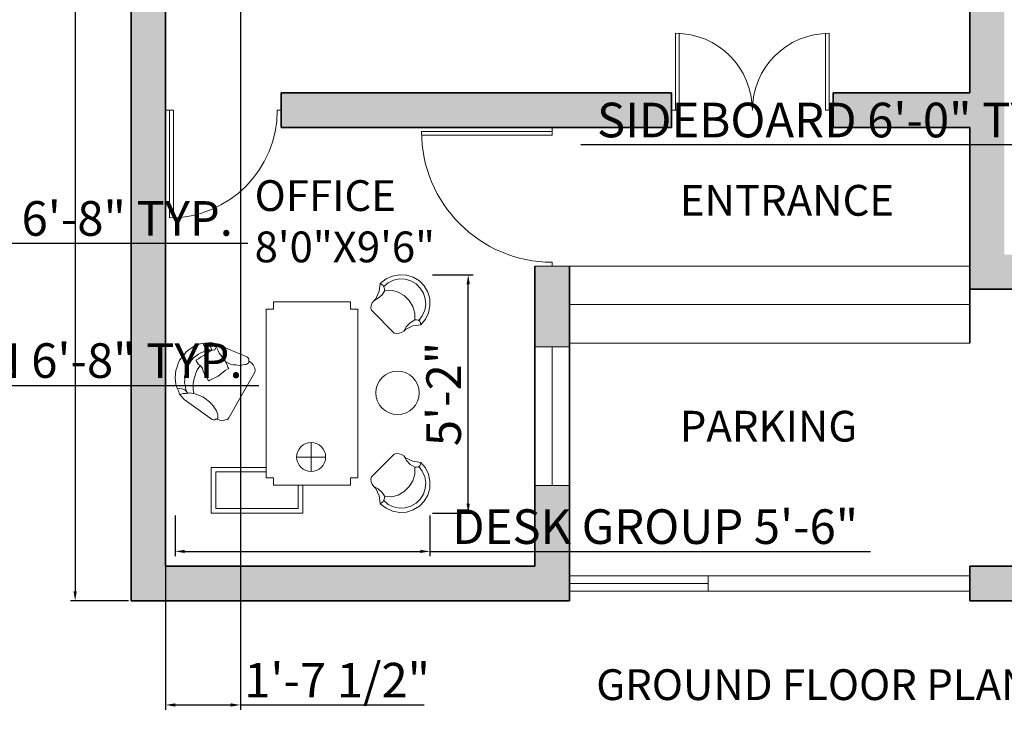
# Model space of a CAD drawing. Units: inches. Extents: x 3592 to 4861, y 1650 to 2243.
# Tile 2 of 30: x 4009 to 4265, y 1650 to 1836. Entities that reach past the tile are written whole.
import ezdxf

# ---------------------------------------------------------------- set-up
doc = ezdxf.new("R2010")
doc.units = ezdxf.units.IN
for name, color, linetype, lineweight in [('A-ANNO-DIMS', 2, 'Continuous', 13), ('A-ANNO-TEXT', 7, 'Continuous', 25), ('A-AREA-IDEN', 7, 'Continuous', 18), ('A-DOOR', 3, 'Continuous', 20), ('A-FLOR-STRS', 7, 'Continuous', 18), ('A-FURN', 9, 'Continuous', 13), ('A-GLAZ', 4, 'Continuous', 18), ('A-WALL', 7, 'Continuous', 35)]:
    doc.layers.add(name, color=color, linetype=linetype, lineweight=lineweight)
doc.layers.add('A-WALL-PATT', color=252, linetype='Continuous', lineweight=13, true_color=0x939598)
doc.styles.get("Standard").update_dxf_attribs({"font": 'arial.ttf'})
doc.dimstyles.new('ISO-25', dxfattribs={"dimtxt": 9, "dimasz": 2.5, "dimexe": 1.25, "dimexo": 0.625, "dimtad": 1, "dimlunit": 3, "dimtxsty": 'Standard', "dimcen": 2.5, "dimadec": 0, "dimazin": 0, "dimtfac": 1, "dimtmove": 0, "dimatfit": 3, "dimfxl": 1, "dimarcsym": 0})

# ---------------------------------------------------------------- blocks, each defined once
blk = doc.blocks.new('2')
for p, q in [((3637.19, 1914.49), (3637.19, 1942.49)), ((3638.19, 1914.49), (3638.19, 1942.49)), ((3636.19, 1914.49), (3638.19, 1914.49)), ((3665.19, 1914.49), (3666.19, 1914.49))]:
    blk.add_line(p, q)
blk.add_arc((3637.19, 1914.49), 28, 0, 90)
blk = doc.blocks.new('1')
for p, q in [((3628.27, 1890.86), (3628.27, 1924.86)), ((3629.27, 1890.86), (3629.27, 1924.86)), ((3627.27, 1890.86), (3629.27, 1890.86)), ((3662.27, 1890.86), (3663.27, 1890.86))]:
    blk.add_line(p, q)
blk.add_arc((3628.27, 1890.86), 34, 0, 90)
blk = doc.blocks.new('MD')
for p, q in [((3665.34, 1831.69), (3665.34, 1851.69)), ((3666.34, 1831.69), (3666.34, 1851.69)), ((3704.34, 1831.69), (3704.34, 1851.69)), ((3705.34, 1831.69), (3705.34, 1851.69)), ((3664.34, 1831.69), (3666.34, 1831.69)), ((3706.34, 1831.69), (3704.34, 1831.69))]:
    blk.add_line(p, q)
for centre, start, end in [((3665.34, 1831.69), 0, 90), ((3705.34, 1831.69), 90, 180)]:
    blk.add_arc(centre, 20, start, end)
blk = doc.blocks.new('*D6')
at = {"layer": 'A-ANNO-DIMS', "color": 0, "lineweight": -2, "transparency": 16777216}
for p, q in [((4037.74, 2165.22), (4022.59, 2165.22)), ((4023.84, 2162.72), (4023.84, 1687.72)), ((4037.74, 1685.22), (4022.59, 1685.22))]:
    blk.add_line(p, q, dxfattribs=at)
at = {"layer": 'A-ANNO-DIMS', "color": 0, "transparency": 16777216}
for points in [[(4023.43, 2162.72), (4024.26, 2162.72), (4023.84, 2165.22)], [(4023.43, 1687.72), (4024.26, 1687.72), (4023.84, 1685.22)]]:
    blk.add_solid(points, dxfattribs=at)
at = {"layer": 'Defpoints', "color": 0, "transparency": 16777216}
for p in [(4038.37, 2165.22), (4023.84, 1685.22), (4038.37, 1685.22)]:
    blk.add_point(p, dxfattribs=at)
at = {"layer": 'A-ANNO-DIMS', "color": 0, "transparency": 16777216, "insert": (4018.62, 1925.22), "char_height": 9, "attachment_point": 5, "rotation": 90}
blk.add_mtext("40'", dxfattribs=at)
blk = doc.blocks.new('desk-20')
at = {"color": 0, "linetype": 'ByBlock'}
for p, q in [((0.2166, 1.9076), (0.1582, 1.8904)), ((0.2792, 1.9099), (0.2166, 1.9076)), ((0.3395, 1.8969), (0.2792, 1.9099)), ((0.3961, 1.8709), (0.3395, 1.8969)), ((1.6928, 1.8709), (1.7493, 1.8969)), ((1.7493, 1.8969), (1.8096, 1.9099)), ((1.8096, 1.9099), (1.8723, 1.9076)), ((1.8723, 1.9076), (1.9307, 1.8904)), ((0.0616, 1.8175), (0.0287, 1.7633)), ((0.1043, 1.8602), (0.0616, 1.8175)), ((0.1238, 1.8255), (0.0875, 1.7892)), ((0.1582, 1.8904), (0.1043, 1.8602)), ((0.167, 1.8534), (0.1238, 1.8255)), ((0.2166, 1.8686), (0.167, 1.8534)), ((0.2662, 1.8732), (0.2166, 1.8686)), ((0.3178, 1.8644), (0.2662, 1.8732)), ((0.3655, 1.8427), (0.3178, 1.8644)), ((0.4064, 1.8125), (0.3655, 1.8427)), ((0.4434, 1.8297), (0.3961, 1.8709)), ((0.4045, 1.8083), (0.4003, 1.7934)), ((0.4129, 1.8213), (0.4045, 1.8083)), ((0.4285, 1.8278), (0.4129, 1.8213)), ((0.4434, 1.8297), (0.4285, 1.8278)), ((0.4434, 1.8297), (0.4537, 1.7591)), ((1.6455, 1.8297), (1.6351, 1.7591)), ((1.6455, 1.8297), (1.6928, 1.8709)), ((1.6455, 1.8297), (1.6604, 1.8278)), ((1.6604, 1.8278), (1.676, 1.8213)), ((1.676, 1.8213), (1.6844, 1.8083)), ((1.6825, 1.8125), (1.7234, 1.8427)), ((1.6844, 1.8083), (1.6886, 1.7934)), ((1.7234, 1.8427), (1.7711, 1.8644)), ((1.7711, 1.8644), (1.8226, 1.8732)), ((1.8226, 1.8732), (1.8723, 1.8686)), ((1.8723, 1.8686), (1.9219, 1.8534)), ((1.9219, 1.8534), (1.9651, 1.8255)), ((1.9307, 1.8904), (1.9845, 1.8602)), ((1.9651, 1.8255), (2.0013, 1.7892)), ((1.9845, 1.8602), (2.0273, 1.8175)), ((2.0273, 1.8175), (2.0601, 1.7633)), ((0.0287, 1.7633), (0.0096, 1.7052)), ((0.0612, 1.7438), (0.0463, 1.6945)), ((0.0875, 1.7892), (0.0612, 1.7438)), ((0.2315, 1.7285), (0.1887, 1.6857)), ((0.2834, 1.7606), (0.2315, 1.7285)), ((0.3418, 1.7762), (0.2834, 1.7606)), ((0.4022, 1.7785), (0.3418, 1.7762)), ((0.4003, 1.7934), (0.4022, 1.7785)), ((0.4022, 1.7785), (0.4258, 1.7373)), ((0.4258, 1.7373), (0.4602, 1.7052)), ((0.4537, 1.7591), (0.4843, 1.6964)), ((1.6351, 1.7591), (1.6046, 1.6964)), ((1.663, 1.7373), (1.6287, 1.7052)), ((1.6867, 1.7785), (1.663, 1.7373)), ((1.6886, 1.7934), (1.6867, 1.7785)), ((1.6867, 1.7785), (1.747, 1.7762)), ((1.747, 1.7762), (1.8054, 1.7606)), ((1.8054, 1.7606), (1.8574, 1.7285)), ((1.8574, 1.7285), (1.9001, 1.6857)), ((2.0013, 1.7892), (2.0277, 1.7438)), ((2.0277, 1.7438), (2.0426, 1.6945)), ((2.0601, 1.7633), (2.0792, 1.7052)), ((0.0096, 1.7052), (0.0073, 1.6426)), ((0.0073, 1.6426), (0.0184, 1.5819)), ((0.0463, 1.6945), (0.0444, 1.6422)), ((0.0444, 1.6422), (0.0551, 1.5926)), ((0.1887, 1.6857), (0.1586, 1.6334)), ((0.4602, 1.7052), (0.5011, 1.6812)), ((0.5011, 1.6812), (0.4843, 1.6964)), ((0.5121, 1.6617), (0.5011, 1.6812)), ((0.5186, 1.6399), (0.5121, 1.6617)), ((0.5209, 1.6185), (0.5186, 1.6399)), ((1.5679, 1.6185), (1.5702, 1.6399)), ((1.5702, 1.6399), (1.5767, 1.6617)), ((1.5767, 1.6617), (1.5878, 1.6812)), ((1.6287, 1.7052), (1.5878, 1.6812)), ((1.5878, 1.6812), (1.6046, 1.6964)), ((1.9001, 1.6857), (1.9303, 1.6334)), ((2.0445, 1.6422), (2.0338, 1.5926)), ((2.0426, 1.6945), (2.0445, 1.6422)), ((2.0815, 1.6426), (2.0704, 1.5819)), ((2.0792, 1.7052), (2.0815, 1.6426)), ((0.0184, 1.5819), (0.044, 1.5258)), ((0.0551, 1.5926), (0.0765, 1.5452)), ((0.1586, 1.6334), (0.1433, 1.5754)), ((0.1433, 1.5754), (0.1452, 1.5154)), ((0.5163, 1.5972), (0.3174, 1.3982)), ((0.5163, 1.5972), (0.5209, 1.6185)), ((1.5725, 1.5972), (1.5679, 1.6185)), ((1.5725, 1.5972), (1.7715, 1.3982)), ((1.9303, 1.6334), (1.9456, 1.5754)), ((1.9456, 1.5754), (1.9437, 1.5154)), ((2.0338, 1.5926), (2.0124, 1.5452)), ((2.0704, 1.5819), (2.0449, 1.5258)), ((0.044, 1.5258), (0.0829, 1.4761)), ((0.0765, 1.5452), (0.1108, 1.5063)), ((0.0982, 1.4975), (0.0829, 1.4761)), ((0.1517, 1.4654), (0.0829, 1.4761)), ((0.1196, 1.5105), (0.0982, 1.4975)), ((0.1452, 1.5154), (0.1196, 1.5105)), ((0.1818, 1.4918), (0.1452, 1.5154)), ((0.2166, 1.4356), (0.1517, 1.4654)), ((0.212, 1.457), (0.1818, 1.4918)), ((1.8723, 1.4356), (1.9372, 1.4654)), ((1.8769, 1.457), (1.907, 1.4918)), ((1.907, 1.4918), (1.9437, 1.5154)), ((1.9372, 1.4654), (2.0059, 1.4761)), ((1.9437, 1.5154), (1.9693, 1.5105)), ((1.9693, 1.5105), (1.9906, 1.4975)), ((2.0124, 1.5452), (1.978, 1.5063)), ((1.9906, 1.4975), (2.0059, 1.4761)), ((2.0449, 1.5258), (2.0059, 1.4761)), ((0.2342, 1.4181), (0.212, 1.457)), ((0.2166, 1.4356), (0.2342, 1.4181)), ((0.2342, 1.4181), (0.2532, 1.4051)), ((0.2532, 1.4051), (0.275, 1.3963)), ((0.275, 1.3963), (0.2983, 1.3944)), ((0.2983, 1.3944), (0.3174, 1.3982)), ((1.7906, 1.3944), (1.7715, 1.3982)), ((1.8138, 1.3963), (1.7906, 1.3944)), ((1.8356, 1.4051), (1.8138, 1.3963)), ((1.8547, 1.4181), (1.8356, 1.4051)), ((1.8547, 1.4181), (1.8769, 1.457)), ((1.8723, 1.4356), (1.8547, 1.4181)), ((0.3084, 1.2145), (0.2444, 1.2145)), ((0.2444, 1.2145), (0.2444, 0.5425)), ((0.3084, 1.2785), (0.3084, 1.2145)), ((1.7804, 1.2785), (0.3084, 1.2785)), ((1.7804, 1.2145), (1.7804, 1.2785)), ((1.8444, 1.2145), (1.7804, 1.2145)), ((1.8444, 0.5425), (1.8444, 1.2145)), ((0.4901, 0.7453), (0.4901, 0.9986)), ((0.6167, 0.8719), (0.3635, 0.8719)), ((0.2444, 0.8), (0, 0.8)), ((0, 0.8), (0, 0)), ((0.2444, 0.76), (0.04, 0.76)), ((0.04, 0.76), (0.04, 0.04)), ((0.2444, 0.5425), (0.3084, 0.5425)), ((0.3084, 0.5425), (0.3084, 0.4785)), ((1.7804, 0.4785), (1.7804, 0.5425)), ((1.7804, 0.5425), (1.8444, 0.5425)), ((0.3084, 0.4785), (1.7804, 0.4785)), ((0.36, 0.04), (0.36, 0.4785)), ((0.4, 0), (0.4, 0.4785)), ((1.2309, 0.3814), (0.831, 0.1524)), ((0.831, 0.1524), (1.2309, 0.3814)), ((1.2309, 0.3814), (1.2494, 0.3818)), ((1.2309, 0.3814), (1.2494, 0.3818)), ((1.2494, 0.3818), (1.2673, 0.3798)), ((1.2494, 0.3818), (1.2673, 0.3798)), ((1.2673, 0.3798), (1.2823, 0.3718)), ((1.2673, 0.3798), (1.2823, 0.3718)), ((1.2823, 0.3718), (1.2955, 0.3671)), ((1.2823, 0.3718), (1.2955, 0.3671)), ((1.2955, 0.3671), (1.3075, 0.3573)), ((1.2955, 0.3671), (1.3075, 0.3573)), ((1.3075, 0.3573), (1.3196, 0.3436)), ((1.3075, 0.3573), (1.3196, 0.3436)), ((1.2931, 0.2677), (1.2906, 0.2433)), ((1.2971, 0.2929), (1.2931, 0.2677)), ((1.2988, 0.3043), (1.2971, 0.2929)), ((1.3007, 0.3117), (1.2988, 0.3043)), ((1.3076, 0.3178), (1.3007, 0.3117)), ((1.3104, 0.3236), (1.3076, 0.3178)), ((1.3191, 0.3266), (1.3104, 0.3236)), ((1.3262, 0.3287), (1.3191, 0.3266)), ((1.3196, 0.3436), (1.3262, 0.3287)), ((1.3196, 0.3436), (1.3262, 0.3287)), ((1.3392, 0.3279), (1.3262, 0.3287)), ((1.3262, 0.3287), (1.3392, 0.3279)), ((1.3441, 0.3266), (1.3392, 0.3279)), ((1.3392, 0.3279), (1.3441, 0.3266)), ((1.3515, 0.3247), (1.3441, 0.3266)), ((1.3441, 0.3266), (1.3515, 0.3247)), ((1.3582, 0.3203), (1.3515, 0.3247)), ((1.3515, 0.3247), (1.3582, 0.3203)), ((1.3637, 0.3109), (1.3582, 0.3203)), ((1.3582, 0.3203), (1.3637, 0.3109)), ((1.4807, 0.0353), (1.3637, 0.3109)), ((1.3637, 0.3109), (1.4807, 0.0353)), ((1.2906, 0.2433), (1.294, 0.2161)), ((1.294, 0.2161), (1.2946, 0.1936)), ((1.2946, 0.1936), (1.302, 0.1666)), ((0.8074, 0.0928), (0.8104, 0.1091)), ((0.8074, 0.0928), (0.8104, 0.1091)), ((0.8091, 0.0792), (0.8074, 0.0928)), ((0.8091, 0.0792), (0.8074, 0.0928)), ((0.8104, 0.1091), (0.8137, 0.1214)), ((0.8104, 0.1091), (0.8137, 0.1214)), ((0.8137, 0.1214), (0.8173, 0.1402)), ((0.8137, 0.1214), (0.8173, 0.1402)), ((0.8173, 0.1402), (0.831, 0.1524)), ((0.8173, 0.1402), (0.831, 0.1524)), ((1.2452, 0.121), (1.196, 0.059)), ((1.2452, 0.121), (1.2633, 0.1544)), ((1.2633, 0.1544), (1.2752, 0.1447)), ((1.2752, 0.1447), (1.2859, 0.1406)), ((1.3249, 0.1237), (1.2859, 0.1406)), ((1.302, 0.1666), (1.3216, 0.1259)), ((1.3638, 0.0964), (1.3249, 0.1237)), ((1.3971, 0.0679), (1.3638, 0.0964)), ((0, 0), (0.4, 0)), ((0.04, 0.04), (0.36, 0.04)), ((0.8169, 0.0587), (0.8091, 0.0792)), ((0.8169, 0.0587), (0.8091, 0.0792)), ((0.8138, 0.0319), (0.8118, 0.0245)), ((0.8118, 0.0245), (0.8138, 0.0319)), ((0.8118, 0.0245), (0.8155, 0.0183)), ((0.8155, 0.0183), (0.8118, 0.0245)), ((0.8206, 0.038), (0.8138, 0.0319)), ((0.8138, 0.0319), (0.8206, 0.038)), ((0.8155, 0.0183), (0.8178, 0.0072)), ((0.8178, 0.0072), (0.8155, 0.0183)), ((0.8208, 0.0485), (0.8169, 0.0587)), ((0.8208, 0.0485), (0.8169, 0.0587)), ((0.8178, 0.0072), (0.9916, -0.2373)), ((0.9916, -0.2373), (0.8178, 0.0072)), ((0.8208, 0.0485), (0.8206, 0.038)), ((0.8206, 0.038), (0.8208, 0.0485)), ((0.8261, 0.0537), (0.8208, 0.0485)), ((0.8348, 0.0567), (0.8261, 0.0537)), ((0.8444, 0.0581), (0.8348, 0.0567)), ((0.8549, 0.058), (0.8444, 0.0581)), ((0.8613, 0.0576), (0.8549, 0.058)), ((0.8681, 0.0532), (0.8613, 0.0576)), ((0.8936, 0.0451), (0.8681, 0.0532)), ((0.9113, 0.0326), (0.8936, 0.0451)), ((0.9358, 0.0156), (0.9113, 0.0326)), ((0.956, 0.0024), (0.9358, 0.0156)), ((0.9734, -0.0167), (0.956, 0.0024)), ((1.196, 0.059), (1.1611, -0.0135)), ((1.3971, 0.0679), (1.4186, 0.0596)), ((1.4217, 0.0114), (1.4121, -0.0151)), ((1.4186, 0.0596), (1.4462, 0.0444)), ((1.4211, 0.0089), (1.4385, 0.0004)), ((1.4238, 0.0043), (1.4213, -0.0201)), ((1.4217, 0.0114), (1.4262, 0.0286)), ((1.4433, 0.0386), (1.4231, 0.0268)), ((1.4273, -0.0125), (1.4238, 0.0043)), ((1.4385, 0.0004), (1.465, -0.0092)), ((1.4462, 0.0444), (1.4433, 0.0386)), ((1.4865, 0.0075), (1.4807, 0.0353)), ((1.4807, 0.0353), (1.4865, 0.0075)), ((1.4876, -0.0231), (1.4865, 0.0075)), ((1.4865, 0.0075), (1.4876, -0.0231)), ((1.0007, -0.0528), (0.9734, -0.0167)), ((1.015, -0.0737), (1.0007, -0.0528)), ((1.0237, -0.0957), (1.015, -0.0737)), ((1.1552, -0.0211), (1.1611, -0.0135)), ((1.1554, -0.0251), (1.1552, -0.0211)), ((1.1763, -0.0359), (1.1554, -0.0251)), ((1.1911, -0.0398), (1.1763, -0.0359)), ((1.1911, -0.0398), (1.2124, -0.0586)), ((1.2124, -0.0586), (1.2367, -0.0715)), ((1.2367, -0.0715), (1.2653, -0.0777)), ((1.2934, -0.1009), (1.2653, -0.0777)), ((1.3766, -0.0649), (1.3636, -0.0892)), ((1.392, -0.0414), (1.3766, -0.0649)), ((1.4121, -0.0151), (1.392, -0.0414)), ((1.409, -0.0669), (1.4001, -0.0908)), ((1.417, -0.0414), (1.409, -0.0669)), ((1.4213, -0.0201), (1.417, -0.0414)), ((1.4332, -0.0298), (1.4273, -0.0125)), ((1.4441, -0.0485), (1.4332, -0.0298)), ((1.4646, -0.0657), (1.4441, -0.0485)), ((1.4803, -0.0712), (1.4646, -0.0657)), ((1.465, -0.0092), (1.4889, -0.0182)), ((1.4717, -0.1137), (1.4804, -0.0857)), ((1.4804, -0.0857), (1.4717, -0.1137)), ((1.4804, -0.0857), (1.4841, -0.0564)), ((1.4841, -0.0564), (1.4804, -0.0857)), ((1.4841, -0.0564), (1.4876, -0.0231)), ((1.4876, -0.0231), (1.4841, -0.0564)), ((1.0332, -0.1193), (1.0237, -0.0957)), ((1.0419, -0.1413), (1.0332, -0.1193)), ((1.0471, -0.1717), (1.0419, -0.1413)), ((1.076, -0.1569), (1.0458, -0.1516)), ((1.0493, -0.1933), (1.0471, -0.1717)), ((1.1059, -0.1582), (1.076, -0.1569)), ((1.1334, -0.1588), (1.1059, -0.1582)), ((1.1637, -0.1537), (1.1334, -0.1588)), ((1.1938, -0.1445), (1.1637, -0.1537)), ((1.2238, -0.1353), (1.1938, -0.1445)), ((1.2505, -0.1239), (1.2238, -0.1353)), ((1.2729, -0.1087), (1.2505, -0.1239)), ((1.2891, -0.0972), (1.2729, -0.1087)), ((1.2989, -0.1103), (1.2934, -0.1009)), ((1.3123, -0.1191), (1.2989, -0.1103)), ((1.3359, -0.1345), (1.3123, -0.1191)), ((1.3557, -0.1542), (1.3351, -0.1725)), ((1.3482, -0.1127), (1.3359, -0.1345)), ((1.3526, -0.106), (1.3482, -0.1127)), ((1.3636, -0.0892), (1.3526, -0.106)), ((1.3699, -0.1355), (1.3557, -0.1542)), ((1.3868, -0.1111), (1.3699, -0.1355)), ((1.4001, -0.0908), (1.3868, -0.1111)), ((1.4262, -0.1964), (1.446, -0.1661)), ((1.446, -0.1661), (1.4262, -0.1964)), ((1.446, -0.1661), (1.4599, -0.1435)), ((1.4599, -0.1435), (1.446, -0.1661)), ((1.4599, -0.1435), (1.4717, -0.1137)), ((1.4717, -0.1137), (1.4599, -0.1435)), ((0.9916, -0.2373), (1.0164, -0.2583)), ((1.0164, -0.2583), (0.9916, -0.2373)), ((1.0375, -0.2731), (1.0446, -0.246)), ((1.0446, -0.246), (1.0462, -0.2201)), ((1.0703, -0.2186), (1.0452, -0.2041)), ((1.0452, -0.2041), (1.062, -0.2151)), ((1.0479, -0.2058), (1.0452, -0.2041)), ((1.0452, -0.2041), (1.0479, -0.2056)), ((1.0462, -0.2201), (1.0493, -0.1933)), ((1.0479, -0.2056), (1.0479, -0.2058)), ((1.062, -0.2151), (1.076, -0.2319)), ((1.0949, -0.225), (1.0703, -0.2186)), ((1.076, -0.2319), (1.0847, -0.2539)), ((1.0847, -0.2539), (1.0884, -0.2747)), ((1.1162, -0.2293), (1.0949, -0.225)), ((1.1423, -0.2349), (1.1162, -0.2293)), ((1.1695, -0.2315), (1.1423, -0.2349)), ((1.1955, -0.2331), (1.1695, -0.2315)), ((1.2184, -0.226), (1.1955, -0.2331)), ((1.2472, -0.2217), (1.2184, -0.226)), ((1.2698, -0.2106), (1.2472, -0.2217)), ((1.2925, -0.1994), (1.2698, -0.2106)), ((1.3127, -0.1876), (1.2925, -0.1994)), ((1.3351, -0.1725), (1.3127, -0.1876)), ((1.36, -0.258), (1.3837, -0.2379)), ((1.3837, -0.2379), (1.36, -0.258)), ((1.3837, -0.2379), (1.4099, -0.2185)), ((1.4099, -0.2185), (1.3837, -0.2379)), ((1.4099, -0.2185), (1.4262, -0.1964)), ((1.4262, -0.1964), (1.4099, -0.2185)), ((1.0164, -0.2583), (1.0393, -0.2762)), ((1.0393, -0.2762), (1.0164, -0.2583)), ((1.0393, -0.2762), (1.0682, -0.2865)), ((1.0682, -0.2865), (1.0393, -0.2762)), ((1.0682, -0.2865), (1.0974, -0.3007)), ((1.0974, -0.3007), (1.0682, -0.2865)), ((1.0884, -0.2747), (1.0857, -0.295)), ((1.0974, -0.3007), (1.1229, -0.3087)), ((1.1229, -0.3087), (1.0974, -0.3007)), ((1.1229, -0.3087), (1.1562, -0.3123)), ((1.1562, -0.3123), (1.1229, -0.3087)), ((1.1562, -0.3123), (1.183, -0.3154)), ((1.183, -0.3154), (1.1562, -0.3123)), ((1.183, -0.3154), (1.2192, -0.313)), ((1.2192, -0.313), (1.183, -0.3154)), ((1.2192, -0.313), (1.2464, -0.3097)), ((1.2464, -0.3097), (1.2192, -0.313)), ((1.2464, -0.3097), (1.2786, -0.2971)), ((1.2786, -0.2971), (1.2464, -0.3097)), ((1.2786, -0.2971), (1.3056, -0.2897)), ((1.3056, -0.2897), (1.2786, -0.2971)), ((1.3056, -0.2897), (1.3354, -0.2765)), ((1.3354, -0.2765), (1.3056, -0.2897)), ((1.3354, -0.2765), (1.36, -0.258)), ((1.36, -0.258), (1.3354, -0.2765))]:
    blk.add_line(p, q, dxfattribs=at)
blk.add_circle((1.0505, 1.6265), 0.19, dxfattribs=at)
at = {"color": 0, "linetype": 'ByBlock', "extrusion": (0, 0, -1)}
blk.add_ellipse((0.4901, 0.8719), major_axis=(-0.0895, 0.0895), ratio=1, dxfattribs=at)
blk = doc.blocks.new('GATE-PARKING-104')
for p, q in [((104, 4), (0, 4)), ((36, 0), (36, 4)), ((36, 2), (0, 2)), ((104, 0), (0, 0))]:
    blk.add_line(p, q)
blk = doc.blocks.new('*D146')
at = {"layer": 'A-ANNO-DIMS', "color": 0, "lineweight": -2, "transparency": 16777216}
for p, q in [((3853.06, 1729.84), (3853.06, 1742.47)), ((3855.56, 1741.22), (3930.56, 1741.22)), ((3933.06, 1729.84), (3933.06, 1742.47)), ((3933.06, 1741.22), (4071.6, 1741.22))]:
    blk.add_line(p, q, dxfattribs=at)
at = {"layer": 'A-ANNO-DIMS', "color": 0, "transparency": 16777216}
for points in [[(3855.56, 1741.64), (3855.56, 1740.8), (3853.06, 1741.22)], [(3930.56, 1741.64), (3930.56, 1740.8), (3933.06, 1741.22)]]:
    blk.add_solid(points, dxfattribs=at)
at = {"layer": 'Defpoints', "color": 0, "transparency": 16777216}
for p in [(3933.06, 1741.22), (3853.06, 1729.22), (3933.06, 1729.22)]:
    blk.add_point(p, dxfattribs=at)
at = {"layer": 'A-ANNO-DIMS', "color": 0, "transparency": 16777216, "insert": (4003.58, 1746.5), "char_height": 9, "attachment_point": 5}
blk.add_mtext('LOWER RUN 6\'-8" TYP.', dxfattribs=at)
blk = doc.blocks.new('*D148')
at = {"layer": 'A-ANNO-DIMS', "color": 0, "lineweight": -2, "transparency": 16777216}
for p, q in [((3853.06, 1766.84), (3853.06, 1779.47)), ((3933.06, 1766.84), (3933.06, 1779.47)), ((3855.56, 1778.22), (3930.56, 1778.22)), ((3933.06, 1778.22), (4068.75, 1778.22))]:
    blk.add_line(p, q, dxfattribs=at)
at = {"layer": 'A-ANNO-DIMS', "color": 0, "transparency": 16777216}
for points in [[(3855.56, 1778.64), (3855.56, 1777.8), (3853.06, 1778.22)], [(3930.56, 1778.64), (3930.56, 1777.8), (3933.06, 1778.22)]]:
    blk.add_solid(points, dxfattribs=at)
at = {"layer": 'Defpoints', "color": 0, "transparency": 16777216}
for p in [(3933.06, 1778.22), (3853.06, 1766.22), (3933.06, 1766.22)]:
    blk.add_point(p, dxfattribs=at)
at = {"layer": 'A-ANNO-DIMS', "color": 0, "transparency": 16777216, "insert": (4002.15, 1783.44), "char_height": 9, "attachment_point": 5}
blk.add_mtext('UPPER RUN 6\'-8" TYP.', dxfattribs=at)
blk = doc.blocks.new('*D156')
at = {"layer": 'A-ANNO-DIMS', "color": 0, "lineweight": -2, "transparency": 16777216}
for p, q in [((4291.39, 1793.56), (4291.39, 1804.98)), ((4363.35, 1793.56), (4363.35, 1804.98)), ((4291.39, 1803.73), (4155.28, 1803.73)), ((4360.85, 1803.73), (4293.89, 1803.73))]:
    blk.add_line(p, q, dxfattribs=at)
at = {"layer": 'A-ANNO-DIMS', "color": 0, "transparency": 16777216}
for points in [[(4293.89, 1804.15), (4293.89, 1803.31), (4291.39, 1803.73)], [(4360.85, 1804.15), (4360.85, 1803.31), (4363.35, 1803.73)]]:
    blk.add_solid(points, dxfattribs=at)
at = {"layer": 'Defpoints', "color": 0, "transparency": 16777216}
for p in [(4291.39, 1803.73), (4291.39, 1792.94), (4363.35, 1792.94)]:
    blk.add_point(p, dxfattribs=at)
at = {"layer": 'A-ANNO-DIMS', "color": 0, "transparency": 16777216, "insert": (4222.08, 1809.01), "char_height": 9, "attachment_point": 5}
blk.add_mtext('SIDEBOARD 6\'-0" TYP.', dxfattribs=at)
blk = doc.blocks.new('*D157')
at = {"layer": 'A-ANNO-DIMS', "color": 0, "lineweight": -2, "transparency": 16777216}
for p, q in [((4290.77, 1792.94), (4279.35, 1792.94)), ((4280.6, 1790.44), (4280.6, 1777.72)), ((4290.77, 1775.22), (4279.35, 1775.22)), ((4280.6, 1775.22), (4280.6, 1696.49))]:
    blk.add_line(p, q, dxfattribs=at)
at = {"layer": 'A-ANNO-DIMS', "color": 0, "transparency": 16777216}
for points in [[(4280.18, 1790.44), (4281.02, 1790.44), (4280.6, 1792.94)], [(4280.18, 1777.72), (4281.02, 1777.72), (4280.6, 1775.22)]]:
    blk.add_solid(points, dxfattribs=at)
at = {"layer": 'Defpoints', "color": 0, "transparency": 16777216}
for p in [(4291.39, 1792.94), (4280.6, 1775.22), (4291.39, 1775.22)]:
    blk.add_point(p, dxfattribs=at)
at = {"layer": 'A-ANNO-DIMS', "color": 0, "transparency": 16777216, "insert": (4275.32, 1734.6), "char_height": 9, "attachment_point": 5, "rotation": 90}
blk.add_mtext('1\'-5 1/2" TYP.', dxfattribs=at)
blk = doc.blocks.new('*D166')
at = {"layer": 'A-ANNO-DIMS', "color": 0, "lineweight": -2, "transparency": 16777216}
for p, q in [((4049.84, 1707.38), (4049.84, 1696.82)), ((4116.08, 1707.38), (4116.08, 1696.82)), ((4052.34, 1698.07), (4113.58, 1698.07)), ((4116.08, 1698.07), (4230.63, 1698.07))]:
    blk.add_line(p, q, dxfattribs=at)
at = {"layer": 'A-ANNO-DIMS', "color": 0, "transparency": 16777216}
for points in [[(4052.34, 1698.49), (4052.34, 1697.66), (4049.84, 1698.07)], [(4113.58, 1698.49), (4113.58, 1697.66), (4116.08, 1698.07)]]:
    blk.add_solid(points, dxfattribs=at)
at = {"layer": 'Defpoints', "color": 0, "transparency": 16777216}
for p in [(4049.84, 1708.01), (4116.08, 1708.01), (4116.08, 1698.07)]:
    blk.add_point(p, dxfattribs=at)
at = {"layer": 'A-ANNO-DIMS', "color": 0, "transparency": 16777216, "insert": (4174.61, 1703.35), "char_height": 9, "attachment_point": 5}
blk.add_mtext('DESK GROUP 5\'-6"', dxfattribs=at)
blk = doc.blocks.new('*D167')
at = {"layer": 'A-ANNO-DIMS', "color": 0, "lineweight": -2, "transparency": 16777216}
for p, q in [((4116.7, 1769.97), (4127.27, 1769.97)), ((4126.02, 1710.51), (4126.02, 1767.47)), ((4116.7, 1708.01), (4127.27, 1708.01))]:
    blk.add_line(p, q, dxfattribs=at)
at = {"layer": 'A-ANNO-DIMS', "color": 0, "transparency": 16777216}
for points in [[(4125.6, 1767.47), (4126.43, 1767.47), (4126.02, 1769.97)], [(4125.6, 1710.51), (4126.43, 1710.51), (4126.02, 1708.01)]]:
    blk.add_solid(points, dxfattribs=at)
at = {"layer": 'Defpoints', "color": 0, "transparency": 16777216}
for p in [(4116.08, 1769.97), (4126.02, 1769.97), (4116.08, 1708.01)]:
    blk.add_point(p, dxfattribs=at)
at = {"layer": 'A-ANNO-DIMS', "color": 0, "transparency": 16777216, "insert": (4120.79, 1738.99), "char_height": 9, "attachment_point": 5, "rotation": 90}
blk.add_mtext('5\'-2"', dxfattribs=at)
blk = doc.blocks.new('*D178')
at = {"layer": 'A-ANNO-DIMS', "color": 0, "lineweight": -2, "transparency": 16777216}
for p, q in [((4047.37, 1941.59), (4047.37, 1656.92)), ((4066.79, 1941.59), (4066.79, 1656.92)), ((4049.87, 1658.17), (4064.29, 1658.17)), ((4066.79, 1658.17), (4114.59, 1658.17))]:
    blk.add_line(p, q, dxfattribs=at)
at = {"layer": 'A-ANNO-DIMS', "color": 0, "transparency": 16777216}
for points in [[(4049.87, 1658.59), (4049.87, 1657.75), (4047.37, 1658.17)], [(4064.29, 1658.59), (4064.29, 1657.75), (4066.79, 1658.17)]]:
    blk.add_solid(points, dxfattribs=at)
at = {"layer": 'Defpoints', "color": 0, "transparency": 16777216}
for p in [(4047.37, 1942.22), (4066.79, 1942.22), (4066.79, 1658.17)]:
    blk.add_point(p, dxfattribs=at)
at = {"layer": 'A-ANNO-DIMS', "color": 0, "transparency": 16777216, "insert": (4091.94, 1663.45), "char_height": 9, "attachment_point": 5}
blk.add_mtext('1\'-7 1/2"', dxfattribs=at)

msp = doc.modelspace()

# ---------------------------------------------------------------- hatches: boundary and pattern name
at = {"layer": 'A-WALL-PATT'}
h = msp.add_hatch(color=256, dxfattribs=at)
h.dxf.hatch_style = 1
h.paths.add_polyline_path([(4398.37, 2165.219), (4038.37, 2165.219), (4038.37, 1993.219), (4047.37, 1993.219), (4047.37, 2156.219), (4191.37, 2156.219), (4191.37, 2150.219), (4195.37, 2150.219), (4195.37, 2156.219), (4256.37, 2156.219), (4256.37, 2150.219), (4265.37, 2150.219), (4265.37, 2156.219), (4389.37, 2156.219), (4389.37, 2114.219), (4398.37, 2114.219)])
h.paths.add_polyline_path([(4265.37, 2102.219), (4256.37, 2102.219), (4256.37, 2096.219), (4195.37, 2096.219), (4195.37, 2102.219), (4191.37, 2102.219), (4191.37, 2020.219), (4195.37, 2020.219), (4195.37, 2087.219), (4256.37, 2087.219), (4256.37, 2020.219), (4306.37, 2020.219), (4306.37, 2024.219), (4265.37, 2024.219)], flags=17)
h.paths.add_polyline_path([(4398.37, 2066.219), (4389.37, 2066.219), (4389.37, 2024.219), (4348.37, 2024.219), (4348.37, 2020.219), (4389.37, 2020.219), (4389.37, 1989.719), (4398.37, 1989.719)])
h.paths.add_polyline_path([(4398.37, 1941.719), (4389.37, 1941.719), (4389.37, 1911.219), (4301.37, 1911.219), (4301.37, 1907.219), (4389.37, 1907.219), (4389.37, 1865.219), (4398.37, 1865.219)])
h.paths.add_polyline_path([(4398.37, 1817.219), (4389.37, 1817.219), (4389.37, 1775.219), (4265.37, 1775.219), (4265.37, 1911.219), (4256.37, 1911.219), (4256.37, 1817.219), (4220.87, 1817.219), (4220.87, 1808.219), (4256.37, 1808.219), (4256.37, 1766.219), (4389.37, 1766.219), (4389.37, 1694.219), (4256.37, 1694.219), (4256.37, 1685.219), (4398.37, 1685.219)])
h.paths.add_polyline_path([(4178.87, 1817.219), (4077.37, 1817.219), (4077.37, 1808.219), (4178.87, 1808.219)])
h.paths.add_polyline_path([(4111.37, 2020.219), (4155.37, 2020.219), (4155.37, 2024.219), (4077.37, 2024.219), (4077.37, 2020.219), (4107.37, 2020.219), (4107.37, 1942.219), (4047.37, 1942.219), (4047.37, 1969.219), (4038.37, 1969.219), (4038.37, 1911.219), (4047.37, 1911.219), (4047.37, 1938.219), (4107.37, 1938.219), (4107.37, 1860.219), (4077.37, 1860.219), (4077.37, 1856.219), (4111.37, 1856.219)])
h.paths.add_polyline_path([(4047.37, 1887.219), (4038.37, 1887.219), (4038.37, 1685.219), (4152.37, 1685.219), (4152.37, 1715.219), (4143.37, 1715.219), (4143.37, 1694.219), (4047.37, 1694.219)])
h.paths.add_polyline_path([(4152.37, 1772.219), (4143.37, 1772.219), (4143.37, 1751.219), (4152.37, 1751.219)], flags=17)

# ---------------------------------------------------------------- linework, layer by layer
at = {"layer": 'A-FLOR-STRS'}
for p, q in [((4256.37, 1772.219), (4143.37, 1772.219)), ((4256.37, 1762.219), (4152.37, 1762.219)), ((4256.37, 1752.219), (4152.37, 1752.219))]:
    msp.add_line(p, q, dxfattribs=at)
at = {"layer": 'A-GLAZ'}
for p, q in [((4143.37, 1751.219), (4152.37, 1751.219)), ((4147.87, 1751.219), (4147.87, 1715.219)), ((4143.37, 1715.219), (4152.37, 1715.219))]:
    msp.add_line(p, q, dxfattribs=at)
at = {"layer": 'A-WALL'}
for p, q in [((4038.37, 1685.219), (4038.37, 2165.219)), ((4047.37, 1694.219), (4047.37, 1938.219)), ((4256.37, 1911.219), (4256.37, 1817.219)), ((4178.87, 1817.219), (4077.37, 1817.219)), ((4077.37, 1808.219), (4077.37, 1817.219)), ((4178.87, 1808.219), (4178.87, 1817.219)), ((4256.37, 1817.219), (4220.87, 1817.219)), ((4220.87, 1808.219), (4220.87, 1817.219)), ((4178.87, 1808.219), (4077.37, 1808.219)), ((4256.37, 1808.219), (4220.87, 1808.219)), ((4256.37, 1808.219), (4256.37, 1752.219)), ((4143.37, 1694.219), (4143.37, 1772.219)), ((4152.37, 1685.219), (4152.37, 1772.219)), ((4389.37, 1766.219), (4256.37, 1766.219)), ((4143.37, 1694.219), (4047.37, 1694.219)), ((4256.37, 1694.219), (4256.37, 1685.219)), ((4389.37, 1694.219), (4256.37, 1694.219)), ((4152.37, 1685.219), (4038.37, 1685.219)), ((4398.37, 1685.219), (4256.37, 1685.219))]:
    msp.add_line(p, q, dxfattribs=at)

# ---------------------------------------------------------------- block references
at = {"layer": 'A-DOOR'}
for name, p in [('MD', (514.534, -18.97)), ('GATE-PARKING-104', (4152.369, 1687.719))]:
    msp.add_blockref(name, p, dxfattribs=at)
at = {"layer": 'A-DOOR', "xscale": -1}
for name, p, rotation in [('2', (411.181, 3727.211), 180), ('1', (6038.734, 5435.486), 90)]:
    msp.add_blockref(name, p, dxfattribs=dict(at, rotation=rotation))
at = {"layer": 'A-FURN', "xscale": -29.76719231739299, "yscale": 29.76719231739299, "zscale": 29.76719231739299, "rotation": 270}
msp.add_blockref('desk-20', (4059.227, 1708.008), dxfattribs=at)

# ---------------------------------------------------------------- texts
at = {"layer": 'A-ANNO-TEXT', "insert": (4159.302, 1667.444), "char_height": 8, "attachment_point": 1}
msp.add_mtext_dynamic_manual_height_columns('GROUND FLOOR PLAN', width=131.60551, gutter_width=12.5, heights=[0], dxfattribs=at)
at = {"layer": 'A-AREA-IDEN', "char_height": 8, "attachment_point": 1}
for s, insert in [('OFFICE\\P8\'0"X9\'6"', (4070.49, 1794.54)), ('ENTRANCE', (4181.015, 1793.311)), ('PARKING', (4181.015, 1734.612))]:
    msp.add_mtext_dynamic_manual_height_columns(s, width=121.44943, gutter_width=12.5, heights=[0], dxfattribs=dict(at, insert=insert))

# ---------------------------------------------------------------- dimensions: what is measured, and where the dimension line sits
at = {"layer": 'A-ANNO-DIMS'}
for base, p1, p2, override, picture, middle in [((4023.842, 1685.219), (4038.37, 2165.219), (4038.37, 1685.219), {"dimclrd": 0, "dimclre": 0, "dimclrt": 0}, '*D6', (4018.622, 1925.219)), ((4126.015, 1769.969), (4116.079, 1708.008), (4116.079, 1769.969), {"dimdec": 1, "dimlfac": 1, "dimrnd": 0, "dimzin": 1, "dimdsep": 46, "dimlunit": 4, "dimfrac": 2}, '*D167', (4120.795, 1738.989))]:
    dim = msp.add_linear_dim(base=base, p1=p1, p2=p2, angle=90, dimstyle='ISO-25', override=override, dxfattribs=at)
    dim.commit()
    dim.dimension.update_dxf_attribs({"geometry": picture, "text_midpoint": middle})
dim = msp.add_linear_dim(base=(4066.788, 1658.169), p1=(4047.37, 1942.219), p2=(4066.788, 1942.219), dimstyle='ISO-25', override={"dimdec": 1, "dimlfac": 1, "dimrnd": 0, "dimzin": 1, "dimdsep": 46, "dimlunit": 4, "dimfrac": 2}, dxfattribs=at)
dim.commit()
dim.dimension.update_dxf_attribs({"geometry": '*D178', "text_midpoint": (4091.938, 1663.447)})
for base, p1, p2, angle, text, picture, middle in [((4291.393, 1803.729), (4363.347, 1792.936), (4291.393, 1792.936), 180, 'SIDEBOARD <> TYP.', '*D156', (4222.085, 1809.01)), ((4280.6, 1775.219), (4291.393, 1792.936), (4291.393, 1775.219), 270, '<> TYP.', '*D157', (4275.321, 1734.602))]:
    dim = msp.add_linear_dim(base=base, p1=p1, p2=p2, angle=angle, text=text, dimstyle='ISO-25', override={"dimdec": 1, "dimlfac": 1, "dimrnd": 0, "dimzin": 1, "dimdsep": 46, "dimlunit": 4, "dimfrac": 2}, dxfattribs=at)
    dim.commit()
    dim.dimension.update_dxf_attribs({"geometry": picture, "text_midpoint": middle})
for base, p1, p2, text, picture, middle in [((3933.061, 1778.219), (3853.061, 1766.219), (3933.061, 1766.219), 'UPPER RUN <> TYP.', '*D148', (4002.155, 1783.439)), ((3933.061, 1741.219), (3853.061, 1729.219), (3933.061, 1729.219), 'LOWER RUN <> TYP.', '*D146', (4003.582, 1746.501)), ((4116.079, 1698.072), (4049.84, 1708.008), (4116.079, 1708.008), 'DESK GROUP <>', '*D166', (4174.607, 1703.354))]:
    dim = msp.add_linear_dim(base=base, p1=p1, p2=p2, text=text, dimstyle='ISO-25', override={"dimdec": 1, "dimlfac": 1, "dimrnd": 0, "dimzin": 1, "dimdsep": 46, "dimlunit": 4, "dimfrac": 2}, dxfattribs=at)
    dim.commit()
    dim.dimension.update_dxf_attribs({"geometry": picture, "text_midpoint": middle})

doc.saveas('drawing.dxf')
